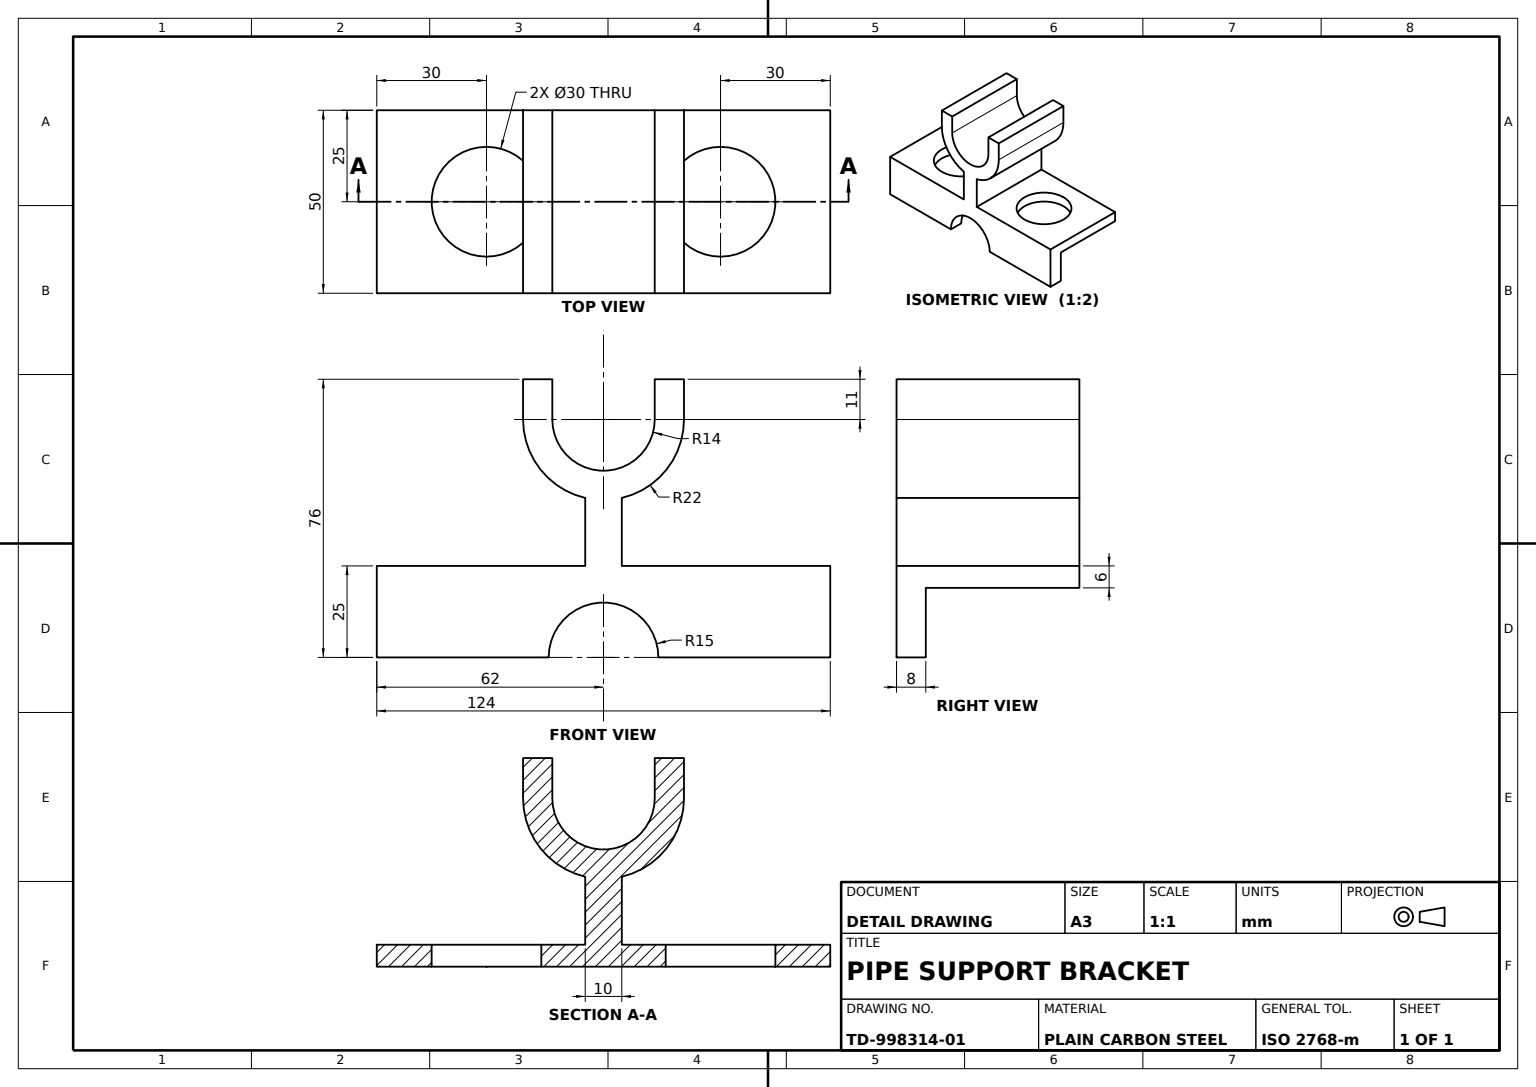
SolidWorks part; units mm, degrees
material "Plain Carbon Steel"
ref_plane "Front Plane" through (0, 0, 0) normal (0, 0, 1) x (1, 0, 0)
ref_plane "Top Plane" through (0, 0, 0) normal (0, 1, 0) x (1, 0, 0)
ref_plane "Right Plane" through (0, 0, 0) normal (1, 0, 0) x (0, 0, -1)
sketch "Bracket Profile Sketch" plane through (0, 0, 0) normal (0, 0, 1) x (1, 0, 0)
  line L1 (-62, 0) -> (-15, 0)
  line L2 (-62, 0) -> (-62, 25)
  line L3 (-62, 25) -> (-5, 25)
  line L4 (62, 0) -> (62, 25)
  line L6 (-5, 43.5757) -> (-5, 25)
  line L7 (5, 43.5757) -> (5, 25)
  line L8 (0, 0) -> (0, 90.2507) construction
  line L9 (5, 25) -> (62, 25)
  line L10 (-22, 65) -> (-22, 76)
  line L11 (-14, 65) -> (-14, 76)
  line L12 (-14, 76) -> (-22, 76)
  line L13 (14, 65) -> (14, 76)
  line L14 (14, 76) -> (22, 76)
  line L15 (22, 65) -> (22, 76)
  line L16 (15, 0) -> (62, 0)
  arc A0 (-14, 65) -> (14, 65) centre (0, 65) ccw
  arc A1 (-22, 65) -> (-5, 43.5757) centre (0, 65) ccw
  arc A2 (5, 43.5757) -> (22, 65) centre (0, 65) ccw
  arc A3 (-22, 65) -> (22, 65) centre (0, 65) ccw construction
  arc A4 (-15, 0) -> (15, 0) centre (0, 0) cw
  point P26 (0, 15)
  dimension "D8" = 15
  dimension "D2" = 10
  dimension "D3" = 28
  dimension "D1" = 8
  dimension "D4" = 11
  dimension "D5" = 40
  dimension "D6" = 25
  dimension "D7" = 124
  dimension "D9" = 62
extrude "Bracket Body" add sketch "Bracket Profile Sketch" along normal mid plane 50
sketch "Cradle Slot Sketch" plane through (62, 0, 0) normal (1, 0, 0) x (0, 0, -1)
  line L0 (-25, 0) -> (-25, 25) construction
  line L1 (25, 0) -> (-17, 0)
  line L2 (25, 0) -> (25, 19)
  line L3 (25, 19) -> (-17, 19)
  line L4 (-17, 0) -> (-17, 19)
  line L5 (-25, 25) -> (25, 25) construction
  dimension "D1" = 8
  dimension "D2" = 6
extrude "Cradle Slot Cut" cut sketch "Cradle Slot Sketch" against normal through all and the other way through all
sketch "Base Cut-Out Sketch" plane through (0, 25, 0) normal (0, 1, 0) x (1, 0, 0)
  line L0 (-62, -25) -> (-62, 25) construction
  line L2 (0, 0) -> (0, 15.7091) construction
  circle A0 centre (-32, 0) radius 15
  circle A1 centre (32, 0) radius 15
  dimension "D1" = 30
  dimension "D2" = 30
extrude "Base Cut-Outs" cut sketch "Base Cut-Out Sketch" against normal through all
